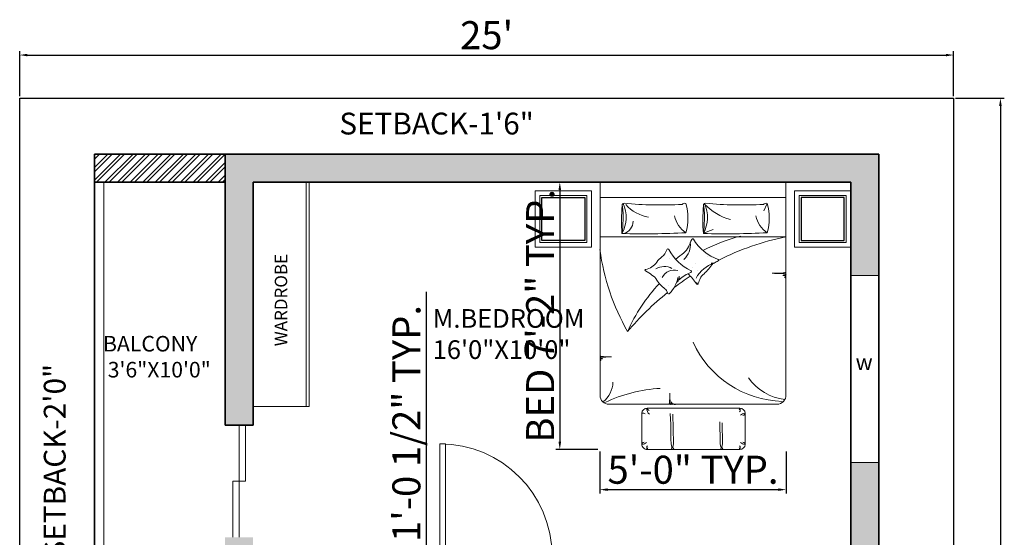
# Model space of a CAD drawing. Units: inches. Extents: x 3488 to 4319, y 780 to 1756.
# Tile 8 of 8: x 3890 to 4206, y 1587 to 1753. Entities that reach past the tile are written whole.
import ezdxf

# ---------------------------------------------------------------- set-up
doc = ezdxf.new("R2010")
doc.units = ezdxf.units.IN
for name, color, linetype, lineweight in [('A-ANNO-IDEN', 7, 'Continuous', 13), ('A-ANNO-TEXT', 7, 'Continuous', 18), ('A-AREA-IDEN', 7, 'Continuous', 18), ('A-DOOR', 4, 'Continuous', 18), ('A-FLOR-CASE', 32, 'Continuous', 18), ('A-FLOR-RAIL', 7, 'Continuous', 20), ('A-WALL', 7, 'Continuous', 35), ('A-WALL-PATT', 252, 'Continuous', 13), ('C-PROP', 7, 'Continuous', 25), ('DIM', 9, 'Continuous', 18), ('FUR', 42, 'Continuous', 18), ('window', 130, 'Continuous', 18)]:
    doc.layers.add(name, color=color, linetype=linetype, lineweight=lineweight)
doc.layers.add('HA-FUR', color=8, linetype='Continuous')
doc.layers.add('wood', color=26, linetype='Continuous')
doc.styles.get("Standard").update_dxf_attribs({"font": 'arial.ttf'})
doc.dimstyles.new('ISO-25', dxfattribs={"dimtxt": 9, "dimasz": 2.5, "dimexe": 1.25, "dimexo": 0.625, "dimtad": 1, "dimdec": 1, "dimlunit": 3, "dimtxsty": 'Standard', "dimcen": 2.5, "dimclrd": 1, "dimclre": 1, "dimclrt": 1, "dimadec": 0, "dimazin": 0, "dimtfac": 1, "dimtdec": 1, "dimtmove": 0, "dimatfit": 3, "dimfxl": 1, "dimarcsym": 0})

# ---------------------------------------------------------------- blocks, each defined once
blk = doc.blocks.new('*U3')
for p, q in [((0, 0), (0, -6)), ((36, 0), (36, -6))]:
    blk.add_line(p, q)
blk.add_lwpolyline([(0, 0), (0, 36), (1.75, 36), (1.75, 0)], close=True)
blk.add_arc((0, 0), 36, 0, 90)
blk = doc.blocks.new('*D7')
at = {"layer": 'Defpoints', "color": 0, "transparency": 16777216}
for p in [(4189.84, 1741.87), (3889.84, 1728.07), (4189.84, 1728.07)]:
    blk.add_point(p, dxfattribs=at)
at = {"layer": 'DIM', "color": 0, "lineweight": -2, "transparency": 16777216}
for p, q in [((3889.84, 1728.69), (3889.84, 1743.12)), ((4189.84, 1728.69), (4189.84, 1743.12)), ((3892.34, 1741.87), (4187.34, 1741.87))]:
    blk.add_line(p, q, dxfattribs=at)
at = {"layer": 'DIM', "color": 0, "transparency": 16777216}
for points in [[(3892.34, 1742.28), (3892.34, 1741.45), (3889.84, 1741.87)], [(4187.34, 1742.28), (4187.34, 1741.45), (4189.84, 1741.87)]]:
    blk.add_solid(points, dxfattribs=at)
at = {"layer": 'DIM', "color": 0, "transparency": 16777216, "insert": (4039.84, 1747.09), "char_height": 9, "attachment_point": 5}
blk.add_mtext("25'", dxfattribs=at)
blk = doc.blocks.new('*D8')
at = {"layer": 'Defpoints', "color": 0, "transparency": 16777216}
for p in [(4189.84, 1728.07), (4189.84, 1308.07), (4204.87, 1308.07)]:
    blk.add_point(p, dxfattribs=at)
at = {"layer": 'DIM', "color": 0, "lineweight": -2, "transparency": 16777216}
for p, q in [((4190.47, 1728.07), (4206.12, 1728.07)), ((4204.87, 1725.57), (4204.87, 1310.57)), ((4190.47, 1308.07), (4206.12, 1308.07))]:
    blk.add_line(p, q, dxfattribs=at)
at = {"layer": 'DIM', "color": 0, "transparency": 16777216}
for points in [[(4204.45, 1725.57), (4205.28, 1725.57), (4204.87, 1728.07)], [(4204.45, 1310.57), (4205.28, 1310.57), (4204.87, 1308.07)]]:
    blk.add_solid(points, dxfattribs=at)
at = {"layer": 'DIM', "color": 0, "transparency": 16777216, "insert": (4199.64, 1518.07), "char_height": 9, "attachment_point": 5, "rotation": 90}
blk.add_mtext("35'", dxfattribs=at)
blk = doc.blocks.new('*X27')
at = {"color": 0}
for p, q in [((3147.8, 8143.4), (3147.8, 8143.4)), ((3155.9, 8182.9), (3155.9, 8182.9)), ((3209.5, 8023.9), (3209.5, 8023.9)), ((3283, 8049.6), (3283, 8049.6)), ((3154.1, 7950.7), (3154.1, 7950.7)), ((3251.6, 7997), (3251.6, 7997))]:
    blk.add_line(p, q, dxfattribs=at)
blk = doc.blocks.new('*X26')
at = {"color": 0}
for p, q in [((3155.9, 8182.9), (3155.9, 8182.9)), ((3139.8, 7939.7), (3139.8, 7939.7))]:
    blk.add_line(p, q, dxfattribs=at)
blk = doc.blocks.new('*X25')
at = {"color": 0}
for p, q in [((3155.9, 8182.9), (3155.9, 8182.9)), ((3139.8, 7939.7), (3139.8, 7939.7))]:
    blk.add_line(p, q, dxfattribs=at)
blk = doc.blocks.new('*X24')
at = {"color": 0}
for p, q in [((3163, 7776.2), (3163, 7776.2)), ((3422.2, 7761.3), (3422.2, 7761.3)), ((3236.2, 7675.7), (3236.2, 7675.7)), ((3244.3, 7698.6), (3244.3, 7698.6)), ((3340.3, 7689.4), (3340.3, 7689.4))]:
    blk.add_line(p, q, dxfattribs=at)
blk = doc.blocks.new('BED1')
for p, q in [((0, -1000), (0, 800)), ((150, 800), (0, 800)), ((150, 800), (150, -1000)), ((2058.7, 800), (150, 800)), ((528, 800), (528, -1000)), ((211.8, 614.9), (277.5, 585.4)), ((2537.2, 404.9), (2237.2, 404.9)), ((2187.2, 354.9), (2187.2, -545.1)), ((2587.2, -545.1), (2587.2, 354.9)), ((2566.3, 178.5), (2565.2, 177.4)), ((2582, 188.1), (2565.4, 174.8)), ((2565.4, 174.8), (2585.7, 165.4)), ((2566.3, -296.8), (2565.2, -297.9)), ((2582, -287.1), (2565.4, -300.5)), ((2565.4, -300.5), (2585.7, -309.9)), ((2237.2, -595.1), (2537.2, -595.1)), ((150, -1000), (0, -1000)), ((150, -1000), (2063.5, -1000))]:
    blk.add_line(p, q)
for points in [[(934, 797.9), (930.9, 797.7), (928.3, 797.4), (926.3, 796.9), (924.9, 796.3), (923.8, 795.6), (923.1, 794.8), (922.7, 793.8), (922.5, 792.7), (922.4, 791.5), (922.5, 790.3), (922.6, 789.2), (922.6, 788.3), (922.6, 787.6), (922.4, 787.3), (922, 787.4), (921.4, 787.9), (920.6, 788.9), (919.5, 790.2), (918.4, 791.6), (917.1, 793.1), (915.9, 794.6), (914.6, 796), (913.3, 797.1), (912.2, 797.9), (911.1, 798.3), (910.1, 798.4), (909.2, 798), (908.3, 797.1), (907.5, 795.8), (906.8, 793.9), (906, 791.4), (905.4, 788.5), (904.8, 785.2), (904.2, 781.7), (903.7, 778.4), (903.2, 775.4), (902.8, 772.9), (902.5, 771.3), (902.3, 770.6), (902.1, 771.2), (902, 772.8), (901.8, 775.2), (901.7, 778.1), (901.5, 781.5), (901.2, 785), (900.8, 788.4), (900.2, 791.5), (899.5, 794.1), (898.6, 796.2), (897.6, 797.9), (896.5, 799.2), (895.3, 800), (894.1, 800.5), (893, 800.7), (891.9, 800.5), (890.9, 800.1), (890, 799), (889.1, 797.1), (888.3, 794), (887.6, 789.3), (886.9, 782.9), (886.2, 774.2), (885.5, 763.1), (884.8, 749.5), (884.2, 734.2), (883.6, 718.3), (883, 702.8), (882.5, 688.8), (882, 677.5), (881.7, 669.8), (881.5, 666.9), (881.3, 669.4), (881.3, 676.7), (881.3, 687.8), (881.2, 701.5), (881.1, 716.8), (880.8, 732.6), (880.2, 748), (879.4, 761.8), (878.3, 773.2), (876.9, 782.2), (875.1, 789.2), (872.9, 794.4), (870.3, 798), (869, 799)], [(2150, -913.5), (2150, 723.2)], [(494.7, 3.1), (458.9, 95.3)], [(2327.6, 182.3), (2530, 185.9), (2550.8, 181.9), (2561.7, 179), (2566, 176.7), (2566.9, 174.4), (2566.3, 171.9), (2562, 169.2), (2550.3, 166.5), (2527.7, 163.9), (2490.6, 161.8), (2345.5, 160.2), (2317.8, 158.5)], [(2149.7, -259.9), (2150, -268.4), (2150.1, -274.1), (2150.1, -278.1), (2150, -281.4), (2149.8, -284), (2149.5, -286.1), (2149.1, -287.8), (2148.7, -289), (2148.1, -289.9), (2147.4, -290.5), (2146.6, -290.8), (2145.6, -291), (2144.6, -291), (2143.6, -291), (2142.7, -290.9), (2141.9, -290.9), (2141.4, -290.9), (2141.1, -291), (2141.2, -291.4), (2141.7, -291.9), (2142.5, -292.6), (2143.5, -293.4), (2144.7, -294.4), (2146, -295.4), (2147.2, -296.5), (2148.4, -297.6), (2149.3, -298.6), (2150, -299.6), (2150.3, -300.5), (2150.4, -301.3), (2150, -302.1), (2149.3, -302.8), (2148.2, -303.5), (2146.6, -304.1), (2144.6, -304.7), (2142.1, -305.2), (2139.3, -305.7), (2136.5, -306.2), (2133.7, -306.6), (2131.2, -307), (2129.2, -307.3), (2127.8, -307.6), (2127.3, -307.8), (2127.7, -308), (2129, -308.1), (2131, -308.2), (2133.5, -308.3), (2136.3, -308.5), (2139.2, -308.7), (2142, -309), (2144.6, -309.5), (2146.8, -310.1), (2148.6, -310.9), (2150, -311.7), (2151, -312.7), (2151.7, -313.6), (2152.1, -314.6), (2152.3, -315.6), (2152.2, -316.5), (2151.8, -317.3), (2150.9, -318.1), (2149.3, -318.8), (2146.7, -319.4), (2142.8, -320), (2137.4, -320.6), (2130.2, -321.2), (2121, -321.8), (2109.7, -322.3), (2096.9, -322.9), (2083.6, -323.4), (2070.7, -323.9), (2059.1, -324.3), (2049.6, -324.7), (2043.2, -325), (2040.8, -325.2), (2042.9, -325.3), (2049, -325.3), (2058.2, -325.3), (2069.6, -325.4), (2082.3, -325.5), (2095.6, -325.8), (2108.4, -326.2), (2119.9, -326.8), (2129.4, -327.8), (2136.9, -329), (2142.7, -330.5), (2147, -332.3), (2150, -334.4), (2150.9, -335.6)], [(2246.5, -294.4), (2530, -289.4), (2550.8, -293.4), (2561.7, -296.3), (2566, -298.6), (2566.9, -300.8), (2566.3, -303.4), (2562, -306.1), (2550.3, -308.8), (2527.7, -311.3), (2490.6, -313.5), (2345.5, -315), (2238.6, -321.8)], [(1733.7, -998.3), (1731.1, -998.1), (1729, -997.8), (1727.4, -997.4), (1726.1, -997), (1725.2, -996.4), (1724.7, -995.7), (1724.3, -994.8), (1724.1, -993.9), (1724.1, -992.9), (1724.1, -991.9), (1724.2, -991), (1724.2, -990.2), (1724.2, -989.7), (1724.1, -989.4), (1723.8, -989.5), (1723.2, -990), (1722.5, -990.8), (1721.7, -991.8), (1720.7, -993), (1719.7, -994.3), (1718.6, -995.5), (1717.5, -996.6), (1716.5, -997.6), (1715.5, -998.3), (1714.6, -998.6), (1713.8, -998.6), (1713, -998.3), (1712.3, -997.6), (1711.7, -996.5), (1711, -994.9), (1710.4, -992.9), (1709.9, -990.4), (1709.4, -987.6), (1708.9, -984.8), (1708.5, -982), (1708.1, -979.5), (1707.8, -977.4), (1707.5, -976.1), (1707.3, -975.5), (1707.1, -976), (1707, -977.3), (1706.9, -979.3), (1706.8, -981.8), (1706.7, -984.6), (1706.4, -987.5), (1706.1, -990.3), (1705.6, -992.9), (1705, -995.1), (1704.2, -996.9), (1703.4, -998.3), (1702.4, -999.3), (1701.5, -1000), (1700.5, -1000.4), (1699.6, -1000.6), (1698.7, -1000.4), (1697.8, -1000.1), (1697, -999.2), (1696.3, -997.6), (1695.7, -995), (1695.1, -991.1), (1694.5, -985.7), (1693.9, -978.5), (1693.3, -969.3), (1692.8, -957.9), (1692.2, -945.2), (1691.7, -931.9), (1691.2, -919), (1690.8, -907.4), (1690.4, -897.9), (1690.1, -891.5), (1689.9, -889.1), (1689.8, -891.2), (1689.8, -897.3), (1689.8, -906.5), (1689.7, -917.9), (1689.6, -930.6), (1689.4, -943.8), (1688.9, -956.6), (1688.3, -968.1), (1687.3, -977.6), (1686.1, -985.2), (1684.6, -991), (1682.8, -995.3), (1680.7, -998.3), (1679.6, -999.2)]]:
    blk.add_lwpolyline(points)
for points in [[(205.5, 619.6, 0.267769), (215.1, 582.4, -0.037739), (204.3, 21.8, 0.684696), (236.7, 5.5, -0.060702), (497.2, 0.1, -0.046649), (225.9, 3.1, -1.318436)], [(489.2, 619.6, 0.144019), (207.6, 617.9, 0.248643)], [(497.2, 0.1, 0.021276), (489.2, 619.6, -0.206383), (326.6, 509.4, 0.237198)], [(211.8, 12.8, 0.143972), (361.6, 262.9, 1.292232)], [(886.4, -150, -0.069098), (985, -66.5, 0.658965), (982.1, -48.7, -0.049789), (927.4, -29, -0.103757), (896.6, -5.4, 0.055725), (800.9, 83.3, -0.11866), (782.7, 104.9, 0.016811), (761.6, 143.9, 0.70791), (748.3, 144, -0.16964), (551.9, -96.6, 0.664036), (554, -110.7, 0.023706), (627, -144.7, -0.134834), (683.2, -188, 0.012748), (746.3, -267.4)], [(205.5, -168.2, 0.267769), (215.1, -205.4, -0.037739), (204.3, -766, 0.684696), (236.7, -782.3, -0.060702), (497.2, -787.7, -0.046649), (225.9, -784.7, -1.318436)], [(489.2, -168.2, 0.144019), (207.6, -169.9, 0.248643)], [(497.2, -787.7, 0.021276), (489.2, -168.2, -0.206383), (326.6, -278.4, 0.237198)], [(969.1, -259.1, 0.263265), (936.3, -236.9, -0.026108), (909.2, -233.2, 0.027613), (945.1, -234.2, -0.089259), (872.7, -120, 0.662242), (857.6, -119.3, -0.162037), (651.8, -332.7, 0.676499), (654, -354.5, -0.160513), (722.9, -401.5, 0.07473), (773.5, -450.3, -0.187721), (845.5, -559.9, 0.70791), (858.8, -561.4, -0.010003), (898.6, -497.3, -0.113819), (947.3, -450.2, 0.099539), (1032.5, -372.4, -0.173425), (1070.9, -346.4, 0.589988), (1076.2, -326.1, 0.137312), (923.9, -245.9, 0.137312)], [(1446, -733.4, -0.095039), (652.8, -1001.7)]]:
    blk.add_lwpolyline(points, format="xyb")
for centre, radius, start, end in [((3208.8, 1363.3), 2739.4, 191.86791, 206.32469), ((1138.6, 793.9), 983.2, 294.60777, 358.30329), ((1608.1, 842.5), 496.3, 305.19014, 354.02057), ((2062.7, 713.7), 86.5, 0, 93.53765), ((2237.2, 354.9), 50, 90, 180), ((2321.1, 409.7), 84.5, 185.61958, 217.13957), ((2227.5, 373.5), 32.8, 17.83305, 72.80048), ((2546.9, 373.5), 32.8, 107.19952, 162.16695), ((2453.3, 409.7), 84.5, 322.86043, 354.38042), ((2537.2, 354.9), 50, 0, 90), ((2098.7, 754.7), 1625, 193.90497, 207.81692), ((2201.9, 323.3), 34.8, 50.8413, 114.9586), ((2212.2, 381.5), 36.5, 226.80948, 258.3841), ((2572.5, 323.3), 34.8, 65.0414, 129.1587), ((2562.2, 381.5), 36.5, 281.6159, 313.19052), ((751.8, 88.7), 34.9, 336.83517, 27.72181), ((684.2, 86), 100.3, 353.675, 10.88198), ((1074.1, 198.8), 306.1, 197.86019, 241.51221), ((341.4, -277.7), 318.5, 60.71255, 115.00895), ((983.7, -79.5), 20.8, 73.79673, 130.45661), ((978.5, -68.6), 14.3, 39.7097, 85.9506), ((602.5, -324), 198.6, 43.20348, 95.05559), ((3208.8, 1363.3), 2739.4, 212.93136, 216.95099), ((981.1, -281.8), 131.1, 164.0372, 243.45361), ((980, -379), 163.4, 152.61037, 209.36102), ((3208.8, 1363.3), 2739.4, 218.63292, 229.94485), ((2098.7, 754.7), 1625, 226.58872, 246.3156), ((3402.5, -342.9), 1408.5, 182.99169, 205.68187), ((-34.4, -471.2), 376.5, 312.01178, 350.96348), ((2178, -513.5), 33, 286.18268, 338.13858), ((2237.2, -545.1), 50, 180, 270), ((2188.1, -476.2), 73, 269.45125, 322.80265), ((2271.1, -580.9), 35.8, 148.90546, 197.55407), ((2453.3, -600), 84.5, 5.61958, 37.13957), ((2537.2, -545.1), 50, 270, 0), ((2572.5, -513.6), 34.8, 230.8413, 294.9586), ((2562.2, -571.8), 36.5, 46.80948, 78.3841), ((2546.9, -563.8), 32.8, 197.83305, 252.80048), ((341.4, -1065.5), 318.5, 60.71255, 115.00895), ((375.7, -807.4), 128.2, 17.40732, 88.51286), ((1929.1, -1126), 250.5, 37.85533, 88.44053), ((2063.5, -913.5), 86.5, 270, 0)]:
    blk.add_arc(centre, radius, start, end)
for name in ['*X26', '*X25', '*X27', '*X24']:
    blk.add_blockref(name, (-2425.3, -8101.4))
blk = doc.blocks.new('A$C647F3D92')
at = {"layer": 'FUR'}
for points in [[(0.6, 0.6), (0, 0.6), (0, 0), (0.6, 0)], [(0.55, 0.55), (0.05, 0.55), (0.05, 0.05), (0.55, 0.05)]]:
    blk.add_lwpolyline(points, close=True, dxfattribs=at)
at = {"layer": 'HA-FUR'}
blk.add_lwpolyline([(0.53, 0.53), (0.07, 0.53), (0.07, 0.07), (0.53, 0.07)], close=True, dxfattribs=at)
blk = doc.blocks.new('A$C38A85F6B')
at = {"layer": 'wood', "xscale": -1, "rotation": 359.9999999999109}
blk.add_blockref('A$C647F3D92', (0.6, 0), dxfattribs=at)
blk = doc.blocks.new('DOOR-SLIDING-36IN')
for p, q in [((2, 0), (2, 36)), ((4, 18), (4, 36)), ((0, 0), (0, 18)), ((0, 18), (4, 18))]:
    blk.add_line(p, q)
blk = doc.blocks.new('*D64')
at = {"layer": 'Defpoints', "color": 0, "transparency": 16777216}
for p in [(4018.59, 1495.91), (4020.5, 1495.91), (4018.59, 1483.17)]:
    blk.add_point(p, dxfattribs=at)
at = {"layer": 'DIM', "color": 1, "lineweight": -2, "transparency": 16777216}
for p, q in [((4020.5, 1495.91), (4020.5, 1665.9)), ((4019.21, 1495.91), (4021.75, 1495.91)), ((4020.5, 1485.67), (4020.5, 1493.41)), ((4019.21, 1483.17), (4021.75, 1483.17))]:
    blk.add_line(p, q, dxfattribs=at)
at = {"layer": 'DIM', "color": 1, "transparency": 16777216}
for points in [[(4020.08, 1493.41), (4020.91, 1493.41), (4020.5, 1495.91)], [(4020.08, 1485.67), (4020.91, 1485.67), (4020.5, 1483.17)]]:
    blk.add_solid(points, dxfattribs=at)
at = {"layer": 'DIM', "color": 1, "transparency": 16777216, "insert": (4015.22, 1582.16), "char_height": 9, "attachment_point": 5, "rotation": 90}
blk.add_mtext('BATH FAUCET 1\'-0 1/2" TYP.', dxfattribs=at)
blk = doc.blocks.new('*D66')
at = {"layer": 'Defpoints', "color": 0, "transparency": 16777216}
for p in [(4076.21, 1701.07), (4063.34, 1615.24), (4076.21, 1615.24)]:
    blk.add_point(p, dxfattribs=at)
at = {"layer": 'DIM', "color": 1, "lineweight": -2, "transparency": 16777216}
for p, q in [((4075.59, 1701.07), (4062.09, 1701.07)), ((4063.34, 1698.57), (4063.34, 1617.74)), ((4075.59, 1615.24), (4062.09, 1615.24))]:
    blk.add_line(p, q, dxfattribs=at)
at = {"layer": 'DIM', "color": 1, "transparency": 16777216}
for points in [[(4062.92, 1698.57), (4063.76, 1698.57), (4063.34, 1701.07)], [(4062.92, 1617.74), (4063.76, 1617.74), (4063.34, 1615.24)]]:
    blk.add_solid(points, dxfattribs=at)
at = {"layer": 'DIM', "color": 1, "transparency": 16777216, "insert": (4058.19, 1658.16), "char_height": 9, "attachment_point": 5, "rotation": 90}
blk.add_mtext('BED 7\'-2" TYP.', dxfattribs=at)
blk = doc.blocks.new('*D67')
at = {"layer": 'Defpoints', "color": 0, "transparency": 16777216}
for p in [(4076.21, 1615.24), (4136.03, 1615.24), (4136.03, 1602.37)]:
    blk.add_point(p, dxfattribs=at)
at = {"layer": 'DIM', "color": 1, "lineweight": -2, "transparency": 16777216}
for p, q in [((4076.21, 1614.62), (4076.21, 1601.12)), ((4136.03, 1614.62), (4136.03, 1601.12)), ((4078.71, 1602.37), (4133.53, 1602.37))]:
    blk.add_line(p, q, dxfattribs=at)
at = {"layer": 'DIM', "color": 1, "transparency": 16777216}
for points in [[(4078.71, 1602.79), (4078.71, 1601.95), (4076.21, 1602.37)], [(4133.53, 1602.79), (4133.53, 1601.95), (4136.03, 1602.37)]]:
    blk.add_solid(points, dxfattribs=at)
at = {"layer": 'DIM', "color": 1, "transparency": 16777216, "insert": (4106.12, 1607.59), "char_height": 9, "attachment_point": 5}
blk.add_mtext('5\'-0" TYP.', dxfattribs=at)

msp = doc.modelspace()

# ---------------------------------------------------------------- hatches: boundary and pattern name
at = {"layer": 'A-WALL-PATT', "transparency": 33554687}
h = msp.add_hatch(color=256, dxfattribs=at)
h.dxf.hatch_style = 1
h.paths.add_polyline_path([(4165.84, 1710.07), (3955.84, 1710.07), (3955.84, 1623.07), (3964.84, 1623.07), (3964.84, 1701.07), (4156.84, 1701.07), (4156.84, 1671.07), (4165.84, 1671.07)])
h.paths.add_polyline_path([(4165.84, 1611.07), (4156.84, 1611.07), (4156.84, 1581.07), (4060.84, 1581.07), (4060.84, 1575.07), (4156.84, 1575.07), (4156.84, 1569.1), (4165.84, 1569.1)])
h.paths.add_polyline_path([(3922.84, 1575.07), (3967.84, 1575.07), (3967.84, 1581.07), (3964.84, 1581.07), (3964.84, 1587.07), (3955.84, 1587.07), (3955.84, 1581.07), (3913.84, 1581.07), (3913.84, 1496.07), (3922.84, 1496.07), (3922.84, 1515.07), (3955.84, 1515.07), (3955.84, 1521.07), (3922.84, 1521.07)])
h.paths.add_polyline_path([(4024.84, 1575.07), (4024.84, 1581.07), (3997.84, 1581.07), (3997.84, 1575.07), (4018.84, 1575.07), (4018.84, 1521.07), (3985.84, 1521.07), (3985.84, 1515.07), (4018.84, 1515.07), (4018.84, 1453.07), (3922.84, 1453.07), (3922.84, 1472.07), (3913.84, 1472.07), (3913.84, 1432.07), (3922.84, 1432.07), (3922.84, 1447.07), (4015.84, 1447.07), (4015.84, 1424.51), (4015.84, 1423.07), (4024.84, 1423.07), (4024.84, 1447.07), (4024.84, 1453.07), (4024.84, 1503.07)])
h.paths.add_polyline_path([(3922.84, 1408.07), (3913.84, 1408.07), (3913.84, 1387.07), (4015.84, 1387.07), (4015.84, 1381.07), (4024.84, 1381.07), (4024.84, 1393.07), (4018.84, 1393.07), (3988.84, 1393.07), (3922.84, 1393.07)])
h.paths.add_polyline_path([(4165.84, 1459.04), (4156.84, 1459.04), (4156.84, 1453.07), (4060.84, 1453.07), (4060.84, 1447.07), (4156.84, 1447.07), (4156.84, 1327.07), (4151.87, 1327.07), (4137.84, 1327.07), (4137.84, 1318.07), (4165.84, 1318.07)])
h.paths.add_polyline_path([(4089.84, 1327.07), (4088.55, 1327.07), (4024.84, 1327.07), (4024.84, 1345.07), (4015.84, 1345.07), (4015.84, 1318.07), (4089.84, 1318.07)])
h.paths.add_polyline_path([(4165.84, 1545.1), (4156.84, 1545.1), (4156.84, 1483.04), (4165.84, 1483.04)])
h = msp.add_hatch(dxfattribs=at)
h.set_pattern_fill('ANSI32', color=256, scale=0.3)
h.set_pattern_definition([(45, (-384.7482, -2.4862), (-2.0205576, 2.0205576), []), (45, (-383.401, -2.4862), (-2.0205576, 2.0205576), [])])
h.paths.add_polyline_path([(3955.84, 1701.07), (3955.84, 1710.07), (3913.84, 1710.07), (3913.84, 1701.07)])

# ---------------------------------------------------------------- linework, layer by layer
at = {"layer": 'A-FLOR-CASE'}
for p, q in [((3981.84, 1701.07), (3981.84, 1629.07)), ((3982.84, 1701.07), (3982.84, 1629.07)), ((3964.84, 1629.07), (3982.84, 1629.07))]:
    msp.add_line(p, q, dxfattribs=at)
at = {"layer": 'A-FLOR-RAIL'}
msp.add_line((3916.84, 1581.07), (3916.84, 1701.07), dxfattribs=at)
at = {"layer": 'A-WALL'}
for p, q in [((3913.84, 1710.07), (4165.84, 1710.07)), ((3913.84, 1387.07), (3913.84, 1710.07)), ((3955.84, 1710.07), (3955.84, 1623.07)), ((4165.84, 1710.07), (4165.84, 1318.07)), ((3913.84, 1701.07), (3955.84, 1701.07)), ((3964.84, 1701.07), (3964.84, 1623.07)), ((3964.84, 1701.07), (4156.84, 1701.07)), ((4156.84, 1701.07), (4156.84, 1581.07)), ((3955.84, 1623.07), (3964.84, 1623.07))]:
    msp.add_line(p, q, dxfattribs=at)
at = {"layer": 'C-PROP'}
for p, q in [((3889.84, 1728.07), (4189.84, 1728.07)), ((3889.84, 1308.07), (3889.84, 1728.07)), ((4189.84, 1728.07), (4189.84, 1308.07))]:
    msp.add_line(p, q, dxfattribs=at)
at = {"layer": 'window'}
for p, q in [((4156.84, 1671.07), (4165.84, 1671.07)), ((4156.84, 1611.07), (4165.84, 1611.07))]:
    msp.add_line(p, q, dxfattribs=at)

# ---------------------------------------------------------------- block references
at = {"layer": 'A-DOOR'}
for name, p in [('DOOR-SLIDING-36IN', (3958.34, 1587.07)), ('*U3', (4024.84, 1581.07))]:
    msp.add_blockref(name, p, dxfattribs=at)
at = {"layer": 'FUR', "xscale": 0.0331718847221821, "yscale": 0.0331718847221821, "zscale": 0.0331718847221821, "rotation": 270}
msp.add_blockref('BED1', (4109.44, 1701.07), dxfattribs=at)
at = {"layer": 'FUR', "yscale": 30.18374333319767, "zscale": 30.18374333319767}
for p, xscale in [((4055.4, 1680.2), 30.18374333319767), ((4156.84, 1680.2), -30.18374333319767)]:
    msp.add_blockref('A$C38A85F6B', p, dxfattribs=dict(at, xscale=xscale))

# ---------------------------------------------------------------- texts
at = {"layer": 'A-ANNO-IDEN'}
msp.add_text('w', height=5, dxfattribs=at).set_placement((4158.36, 1640.79))
at = {"layer": 'A-ANNO-TEXT', "insert": (3992.52, 1723.38), "char_height": 7, "attachment_point": 1}
msp.add_mtext_dynamic_manual_height_columns('\\pxt7;{SETBACK-1\'6"}', width=83.4163, gutter_width=25, heights=[0], dxfattribs=at)
at = {"layer": 'A-ANNO-TEXT', "attachment_point": 1, "rotation": 90}
for s, insert, char_height in [('WARDROBE', (3971.77, 1648.4), 4), ('\\pxt7;{SETBACK-2\'0"}', (3897.59, 1580.28), 7)]:
    msp.add_mtext_dynamic_manual_height_columns(s, width=83.4163, gutter_width=25, heights=[0], dxfattribs=dict(at, insert=insert, char_height=char_height))
at = {"layer": 'A-AREA-IDEN', "attachment_point": 1}
for s, insert, char_height in [('M.BEDROOM\\P16\'0"X10\'0"', (4022.51, 1660.32), 6), ('BALCONY\\P 3\'6"X10\'0"', (3916.6, 1651.71), 5)]:
    msp.add_mtext_dynamic_manual_height_columns(s, width=83.4163, gutter_width=25, heights=[0], dxfattribs=dict(at, insert=insert, char_height=char_height))

# ---------------------------------------------------------------- dimensions: what is measured, and where the dimension line sits
at = {"layer": 'DIM'}
dim = msp.add_linear_dim(base=(4189.84, 1741.87), p1=(3889.84, 1728.07), p2=(4189.84, 1728.07), dimstyle='ISO-25', override={"dimclrd": 0, "dimclre": 0, "dimclrt": 0}, dxfattribs=at)
dim.commit()
dim.dimension.update_dxf_attribs({"geometry": '*D7', "text_midpoint": (4039.84, 1747.09)})
dim = msp.add_linear_dim(base=(4204.87, 1308.07), p1=(4189.84, 1728.07), p2=(4189.84, 1308.07), angle=90, dimstyle='ISO-25', override={"dimclrd": 0, "dimclre": 0, "dimclrt": 0}, dxfattribs=at)
dim.commit()
dim.dimension.update_dxf_attribs({"geometry": '*D8', "text_midpoint": (4199.64, 1518.07)})
for base, p1, p2, angle, text, picture, middle in [((4063.34, 1615.24), (4076.21, 1701.07), (4076.21, 1615.24), 270, 'BED <> TYP.', '*D66', (4058.19, 1658.16)), ((4020.5, 1495.91), (4018.59, 1483.17), (4018.59, 1495.91), 90, 'BATH FAUCET <> TYP.', '*D64', (4015.22, 1582.16))]:
    dim = msp.add_linear_dim(base=base, p1=p1, p2=p2, angle=angle, text=text, dimstyle='ISO-25', override={"dimdec": 1, "dimlfac": 1, "dimrnd": 0, "dimzin": 1, "dimdsep": 46, "dimlunit": 4, "dimfrac": 2}, dxfattribs=at)
    dim.commit()
    dim.dimension.update_dxf_attribs({"geometry": picture, "text_midpoint": middle})
dim = msp.add_linear_dim(base=(4136.03, 1602.37), p1=(4076.21, 1615.24), p2=(4136.03, 1615.24), text='<> TYP.', dimstyle='ISO-25', override={"dimdec": 1, "dimlfac": 1, "dimrnd": 0, "dimzin": 1, "dimdsep": 46, "dimlunit": 4, "dimfrac": 2}, dxfattribs=at)
dim.commit()
dim.dimension.update_dxf_attribs({"geometry": '*D67', "text_midpoint": (4106.12, 1607.59)})

doc.saveas('drawing.dxf')
